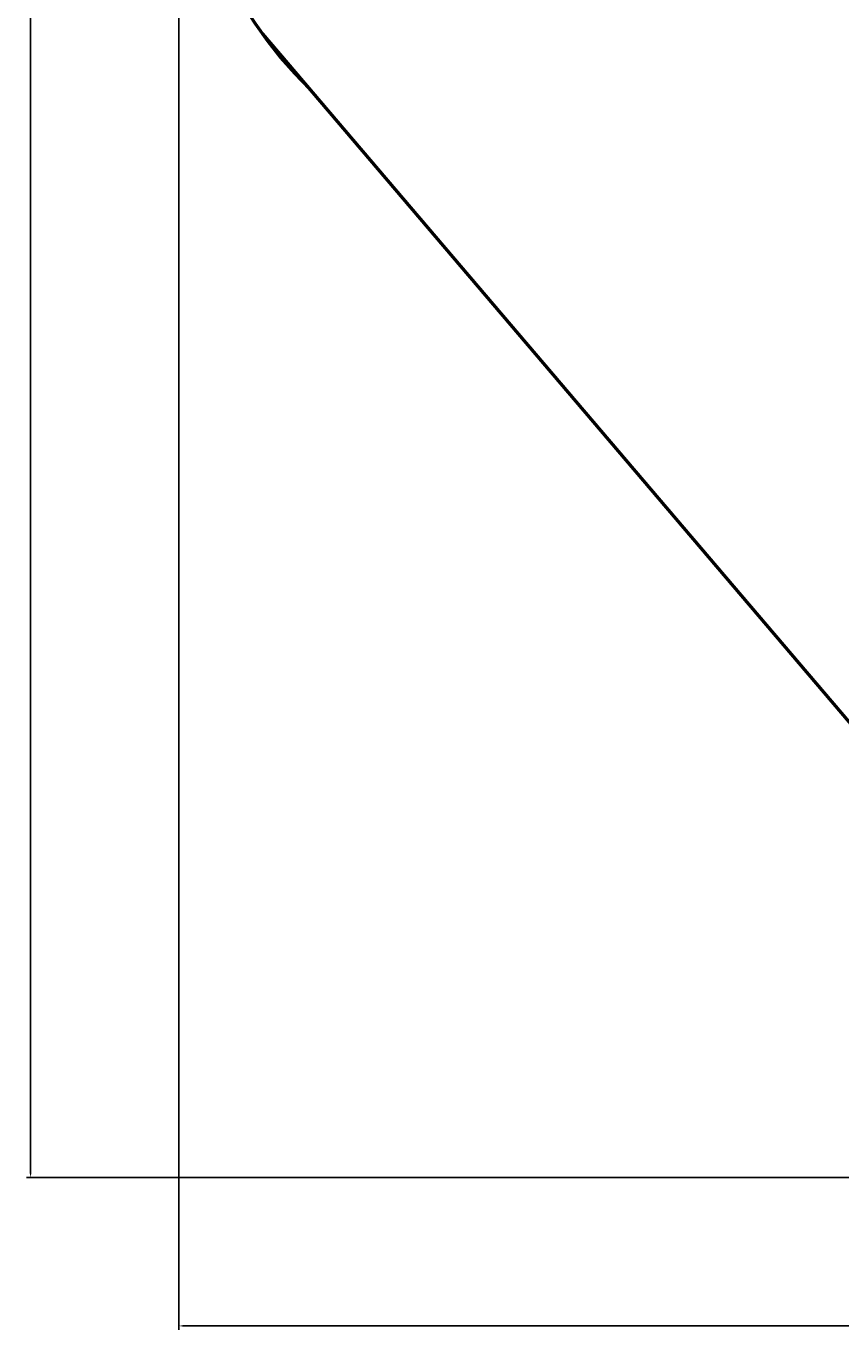
# Model space of a CAD drawing. Units: inches. Extents: x -11 to 126, y -62 to 82.
# Tile 1 of 10: x -8 to 29, y -57 to 1. Entities that reach past the tile are written whole.
import ezdxf

# ---------------------------------------------------------------- set-up
doc = ezdxf.new("R2010")
doc.units = ezdxf.units.IN
doc.header["$MEASUREMENT"] = 0
doc.layers.add('M-DIMS', color=2, linetype='Continuous', lineweight=18)
doc.layers.add('M-OUTL', color=7, linetype='Continuous', lineweight=50)
doc.styles.get("Standard").update_dxf_attribs({"font": 'arial.ttf'})
doc.dimstyles.get("Standard").update_dxf_attribs({"dimtxt": 0.18, "dimasz": 0.18, "dimexe": 0.18, "dimexo": 0.0625, "dimgap": 0.09, "dimtad": 0, "dimtih": 1, "dimtoh": 1, "dimdec": 4, "dimzin": 0, "dimdsep": 46, "dimtxsty": 'Standard', "dimcen": 0.09, "dimadec": 0, "dimazin": 0, "dimtfac": 1, "dimtdec": 4, "dimtofl": 0, "dimtmove": 0, "dimatfit": 3, "dimfxl": 1, "dimtolj": 1, "dimtzin": 0, "dimarcsym": 0})

# ---------------------------------------------------------------- blocks, each defined once
blk = doc.blocks.new('*D5')
at = {"layer": 'Defpoints', "color": 0, "transparency": 16777216}
for p in [(119.232, 12.354), (-0.749, 11.479), (119.232, -57.296)]:
    blk.add_point(p, dxfattribs=at)
at = {"layer": 'M-DIMS', "color": 0, "lineweight": -2, "transparency": 16777216}
for p, q in [((119.232, 12.292), (119.232, -57.476)), ((-0.749, 11.416), (-0.749, -57.476)), ((-0.569, -57.296), (58.786, -57.296)), ((119.052, -57.296), (59.696, -57.296))]:
    blk.add_line(p, q, dxfattribs=at)
at = {"layer": 'M-DIMS', "color": 0, "transparency": 16777216}
for points in [[(-0.569, -57.266), (-0.569, -57.326), (-0.749, -57.296)], [(119.052, -57.266), (119.052, -57.326), (119.232, -57.296)]]:
    blk.add_solid(points, dxfattribs=at)
at = {"layer": 'M-DIMS', "color": 0, "transparency": 16777216, "insert": (59.241, -57.296), "char_height": 0.18, "attachment_point": 5}
blk.add_mtext('\\A1;119.98', dxfattribs=at)
blk = doc.blocks.new('*D6')
at = {"layer": 'Defpoints', "color": 0, "transparency": 16777216}
for p in [(-7.399, 75.354), (59.232, 75.354), (59.232, -50.646)]:
    blk.add_point(p, dxfattribs=at)
at = {"layer": 'M-DIMS', "color": 0, "lineweight": -2, "transparency": 16777216}
for p, q in [((59.169, 75.354), (-7.579, 75.354)), ((-7.399, 75.174), (-7.399, 12.536)), ((-7.399, -50.466), (-7.399, 12.172)), ((59.169, -50.646), (-7.579, -50.646))]:
    blk.add_line(p, q, dxfattribs=at)
at = {"layer": 'M-DIMS', "color": 0, "transparency": 16777216}
for points in [[(-7.429, 75.174), (-7.369, 75.174), (-7.399, 75.354)], [(-7.429, -50.466), (-7.369, -50.466), (-7.399, -50.646)]]:
    blk.add_solid(points, dxfattribs=at)
at = {"layer": 'M-DIMS', "color": 0, "transparency": 16777216, "insert": (-7.399, 12.354), "char_height": 0.18, "attachment_point": 5}
blk.add_mtext('\\A1;126', dxfattribs=at)

msp = doc.modelspace()

# ---------------------------------------------------------------- linework, layer by layer
at = {"layer": 'M-OUTL'}
msp.add_line((3.002, 0.666), (41.77, -44.799), dxfattribs=at)
msp.add_arc((19.232, 12.354), 20, 139.87157, 225.14721, dxfattribs=at)

# ---------------------------------------------------------------- dimensions: what is measured, and where the dimension line sits
at = {"layer": 'M-DIMS'}
dim = msp.add_linear_dim(base=(-7.399, 75.354), p1=(59.232, -50.646), p2=(59.232, 75.354), angle=90, dimstyle='Standard', override={"dimdec": 0, "dimlfac": 1, "dimrnd": 0, "dimzin": 0, "dimdsep": 46, "dimlunit": 2}, dxfattribs=at)
dim.commit()
dim.dimension.update_dxf_attribs({"geometry": '*D6', "text_midpoint": (-7.399, 12.354)})
dim = msp.add_linear_dim(base=(119.232, -57.296), p1=(-0.749, 11.479), p2=(119.232, 12.354), dimstyle='Standard', override={"dimdec": 2, "dimlfac": 1, "dimrnd": 0, "dimzin": 0, "dimdsep": 46, "dimlunit": 2}, dxfattribs=at)
dim.commit()
dim.dimension.update_dxf_attribs({"geometry": '*D5', "text_midpoint": (59.241, -57.296)})

doc.saveas('drawing.dxf')
